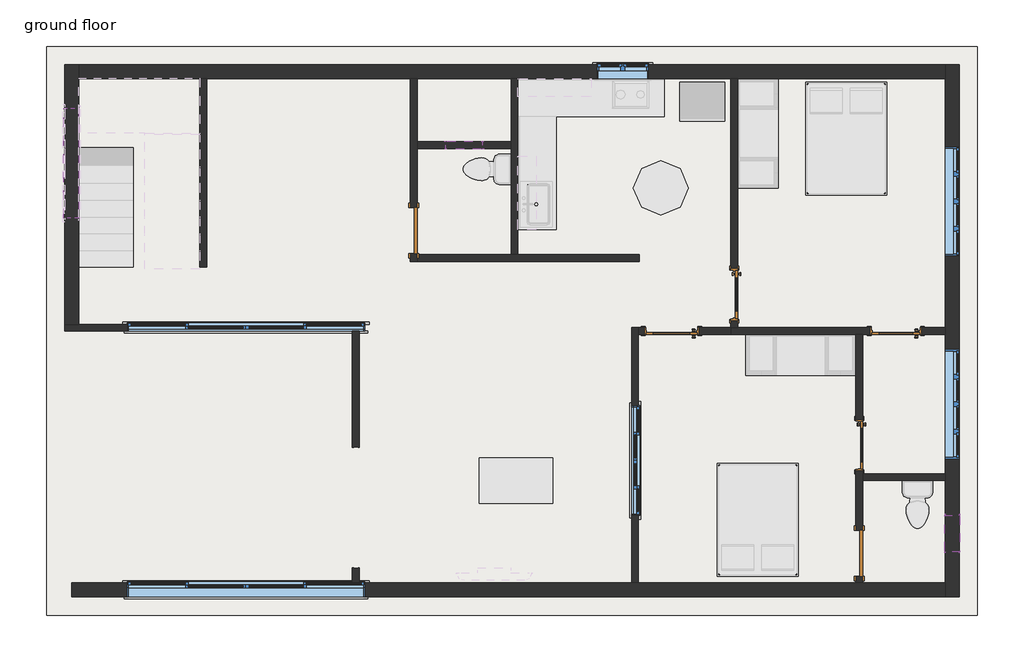
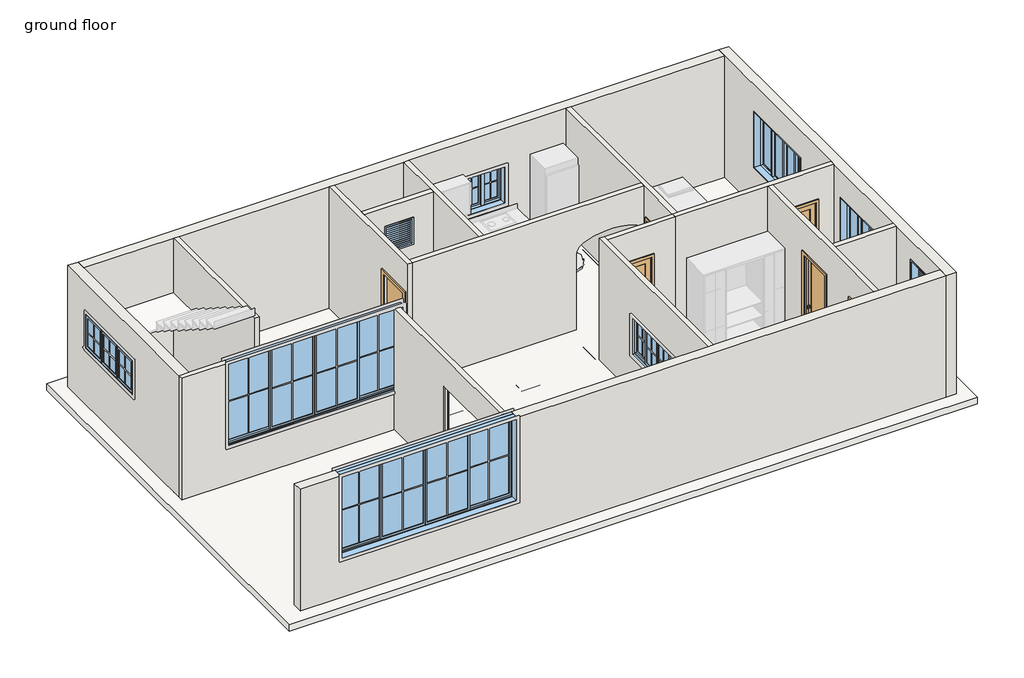
# One storey, part 1 of 2: 17 walls, 9 windows, 7 beams, 6 doors, 1 slab.
"""IFC4 building model written with IfcOpenShell, lengths in millimetres."""

from ifc_helpers import new_model, si_unit, point, frame, origin, place, context, project, spatial, polyline, ellipse_curve, trimmed, outline, extrude, faceted_brep, transform, mapped, element, save
from ifc_brep_helpers import plane_surface, extruded_surface, advanced_brep
from components import door_643e272e, door_51292941, door_214872d5, window_33d4544c, window_339605e1, window_5487fb6d, window_d39e7ecb, window_f2d8fef0, window_cbca41e3, window_8ea0b4a1, window_cd2bb1e7

model = new_model("IFC4")

# Units and contexts
model_context = context("Model", 3, world=origin())
ifc_project = project(units=[si_unit("LENGTHUNIT", "METRE", prefix="MILLI")], contexts=[model_context])

# Site, building, storey
site = spatial("IfcSite", under=ifc_project)
building = spatial("IfcBuilding", under=site)
storey = spatial("IfcBuildingStorey", under=building, Name="ground floor", Elevation=609.6)

# Beams
placement = place(None, origin())
element("IfcBeam", 1, ObjectType="Concrete-Rectangular Beam", at=placement, inside=storey, context=model_context, shape_type="Brep", body=[
    faceted_brep([(-12452.868339, 913.093496, 609.6), (-12452.868339, 684.493496, 609.6), (-8179.318339, 684.493496, 609.6), (-8179.318339, 913.093496, 609.6), (-12452.868339, 913.093496, 304.8), (-8179.318339, 913.093496, 304.8), (-12452.868339, 684.493496, 304.8), (-8179.318339, 684.493496, 304.8)], [[[0, 1, 2, 3]], [[4, 0, 3, 5]], [[6, 4, 5, 7]], [[1, 6, 7, 2]], [[1, 0, 4, 6]], [[3, 2, 7, 5]]]),
    faceted_brep([(1713.981661, 913.093496, 609.6), (1713.981661, 684.493496, 609.6), (1713.981661, 684.493496, 304.8), (1713.981661, 913.093496, 304.8), (-3226.216739, 684.493496, 609.6), (-3226.216739, 913.093496, 609.6), (-3226.216739, 913.093496, 304.8), (-3226.216739, 684.493496, 304.8), (469.381661, 913.093496, 609.6), (240.781661, 913.093496, 609.6), (-1613.418339, 913.093496, 609.6), (-1842.018339, 913.093496, 609.6), (469.381661, 913.093496, 304.8), (240.781661, 913.093496, 304.8), (-1613.418339, 913.093496, 304.8), (-1842.018339, 913.093496, 304.8)], [[[0, 1, 2, 3]], [[4, 5, 6, 7]], [[1, 0, 8, 9, 10, 11, 5, 4]], [[0, 3, 12, 13, 14, 15, 6, 5, 11, 10, 9, 8]], [[3, 2, 7, 6, 15, 14, 13, 12]], [[2, 1, 4, 7]]]),
    faceted_brep([(-7874.518339, 684.493496, 609.6), (-7874.518339, 913.093496, 609.6), (-7874.518339, 913.093496, 304.8), (-7874.518339, 684.493496, 304.8), (-3531.016739, 684.493496, 609.6), (-3531.016739, 913.093496, 609.6), (-5271.018339, 913.093496, 609.6), (-5499.618339, 913.093496, 609.6), (-6947.418339, 913.093496, 609.6), (-7176.018339, 913.093496, 609.6), (-3531.016739, 913.093496, 304.8), (-5271.018339, 913.093496, 304.8), (-5499.618339, 913.093496, 304.8), (-6947.418339, 913.093496, 304.8), (-7176.018339, 913.093496, 304.8), (-3531.016739, 684.493496, 304.8)], [[[0, 1, 2, 3]], [[1, 0, 4, 5, 6, 7, 8, 9]], [[2, 1, 9, 8, 7, 6, 5, 10, 11, 12, 13, 14]], [[3, 2, 14, 13, 12, 11, 10, 15]], [[0, 3, 15, 4]], [[5, 4, 15, 10]]]),
])
element("IfcBeam", 2, ObjectType="Concrete-Rectangular Beam", at=placement, inside=storey, context=model_context, shape_type="SweptSolid", body=[
    extrude(outline(polyline([(-12871.968339, 9244.293496), (-12643.368339, 9244.293496), (-12643.368339, 5415.243496), (-12871.968339, 5415.243496), (-12871.968339, 9244.293496)])), frame((0.0, 0.0, 304.8), z_axis=(0.0, 0.0, 1.0), x_axis=(1.0, 0.0, 0.0)), (0.0, 0.0, 1.0), 304.8),
])
element("IfcBeam", 3, ObjectType="Concrete-Rectangular Beam", at=placement, inside=storey, context=model_context, shape_type="Brep", body=[
    faceted_brep([(-10452.618339, 5110.443496, 609.6), (-10681.218339, 5110.443496, 609.6), (-10681.218339, 5110.443496, 304.8), (-10452.618339, 5110.443496, 304.8), (-10452.618339, 5148.543496, 609.6), (-10452.618339, 5377.143496, 609.6), (-10452.618339, 9282.393496, 609.6), (-10681.218339, 9282.393496, 609.6), (-10681.218339, 5377.143496, 609.6), (-10681.218339, 5148.543496, 609.6), (-10681.218339, 9282.393496, 304.8), (-10681.218339, 5377.143496, 304.8), (-10681.218339, 5148.543496, 304.8), (-10452.618339, 9282.393496, 304.8), (-10452.618339, 5377.143496, 304.8), (-10452.618339, 5148.543496, 304.8)], [[[0, 1, 2, 3]], [[1, 0, 4, 5, 6, 7, 8, 9]], [[2, 1, 9, 8, 7, 10, 11, 12]], [[3, 2, 12, 11, 10, 13, 14, 15]], [[0, 3, 15, 14, 13, 6, 5, 4]], [[7, 6, 13, 10]]]),
])
element("IfcBeam", 4, ObjectType="Concrete-Rectangular Beam", at=placement, inside=storey, context=model_context, shape_type="Brep", body=[
    faceted_brep([(-8274.568339, 5148.543496, 609.6), (-8274.568339, 5339.043496, 609.6), (-7969.768339, 5339.043496, 609.6), (-7969.768339, 5148.543496, 609.6), (-7912.618339, 5148.543496, 609.6), (-7912.618339, 5224.743496, 609.6), (-7912.618339, 5377.143496, 609.6), (-10452.618339, 5377.143496, 609.6), (-10452.618339, 5148.543496, 609.6), (-7969.768339, 5148.543496, 304.8), (-7912.618339, 5148.543496, 304.8), (-8274.568339, 5339.043496, 304.8), (-8274.568339, 5148.543496, 304.8), (-10452.618339, 5148.543496, 304.8), (-10452.618339, 5377.143496, 304.8), (-7912.618339, 5377.143496, 304.8), (-7912.618339, 5224.743496, 304.8), (-7969.768339, 5339.043496, 304.8)], [[[0, 1, 2, 3, 4, 5, 6, 7, 8]], [[3, 9, 10, 4]], [[11, 12, 13, 14, 15, 16, 10, 9, 17]], [[6, 15, 14, 7]], [[11, 1, 0, 12]], [[17, 2, 1, 11]], [[2, 17, 9, 3]], [[8, 7, 14, 13]], [[6, 5, 4, 10, 16, 15]], [[12, 0, 8, 13]]]),
    faceted_brep([(-12643.368339, 5148.543496, 609.6), (-12643.368339, 5377.143496, 609.6), (-12643.368339, 5377.143496, 304.8), (-12643.368339, 5148.543496, 304.8), (-10681.218339, 5377.143496, 609.6), (-10681.218339, 5148.543496, 609.6), (-10681.218339, 5148.543496, 304.8), (-10681.218339, 5377.143496, 304.8)], [[[0, 1, 2, 3]], [[4, 5, 6, 7]], [[1, 0, 5, 4]], [[3, 2, 7, 6]], [[2, 1, 4, 7]], [[0, 3, 6, 5]]]),
])
element("IfcBeam", 5, ObjectType="Concrete-Rectangular Beam", at=placement, inside=storey, context=model_context, shape_type="Brep", body=[
    faceted_brep([(-7912.618339, 5148.543496, 609.6), (-7969.768339, 5148.543496, 609.6), (-7969.768339, 5110.443496, 609.6), (-8141.218339, 5110.443496, 609.6), (-8141.218339, 913.093496, 609.6), (-7912.618339, 913.093496, 609.6), (-7912.618339, 4996.143496, 609.6), (-7912.618339, 5148.543496, 304.8), (-7912.618339, 913.093496, 304.8), (-7912.618339, 4996.143496, 304.8), (-7969.768339, 5148.543496, 304.8), (-8141.218339, 913.093496, 304.8), (-8141.218339, 5110.443496, 304.8), (-7969.768339, 5110.443496, 304.8)], [[[0, 1, 2, 3, 4, 5, 6]], [[7, 0, 6, 5, 8, 9]], [[10, 7, 9, 8, 11, 12, 13]], [[3, 12, 11, 4]], [[0, 7, 10, 1]], [[2, 13, 12, 3]], [[13, 2, 1, 10]], [[5, 4, 11, 8]]]),
])
element("IfcBeam", 6, ObjectType="Concrete-Rectangular Beam", at=placement, inside=storey, context=model_context, shape_type="Brep", body=[
    faceted_brep([(-6947.418339, 9282.393496, 609.6), (-7176.018339, 9282.393496, 609.6), (-7176.018339, 5224.743496, 609.6), (-7176.018339, 4996.143496, 609.6), (-7176.018339, 913.093496, 609.6), (-6947.418339, 913.093496, 609.6), (-6947.418339, 4996.143496, 609.6), (-6947.418339, 5224.743496, 609.6), (-6947.418339, 6215.343496, 609.6), (-6947.418339, 6443.943496, 609.6), (-6947.418339, 8094.943496, 609.6), (-6947.418339, 8323.543496, 609.6), (-7176.018339, 9282.393496, 304.8), (-7176.018339, 5224.743496, 304.8), (-7176.018339, 4996.143496, 304.8), (-7176.018339, 913.093496, 304.8), (-6947.418339, 9282.393496, 304.8), (-6947.418339, 8323.543496, 304.8), (-6947.418339, 8094.943496, 304.8), (-6947.418339, 6443.943496, 304.8), (-6947.418339, 6215.343496, 304.8), (-6947.418339, 5224.743496, 304.8), (-6947.418339, 4996.143496, 304.8), (-6947.418339, 913.093496, 304.8)], [[[0, 1, 2, 3, 4, 5, 6, 7, 8, 9, 10, 11]], [[1, 12, 13, 14, 15, 4, 3, 2]], [[12, 16, 17, 18, 19, 20, 21, 22, 23, 15, 14, 13]], [[16, 0, 11, 10, 9, 8, 7, 6, 5, 23, 22, 21, 20, 19, 18, 17]], [[1, 0, 16, 12]], [[5, 4, 15, 23]]]),
])
element("IfcBeam", 7, ObjectType="Concrete-Rectangular Beam", at=placement, inside=storey, context=model_context, shape_type="Brep", body=[
    faceted_brep([(-5271.018339, 9282.393496, 609.6), (-5499.618339, 9282.393496, 609.6), (-5499.618339, 8323.543496, 609.6), (-5499.618339, 8094.943496, 609.6), (-5499.618339, 6443.943496, 609.6), (-5499.618339, 6215.343496, 609.6), (-5499.618339, 5224.743496, 609.6), (-5499.618339, 4996.143496, 609.6), (-5499.618339, 913.093496, 609.6), (-5271.018339, 913.093496, 609.6), (-5271.018339, 4996.143496, 609.6), (-5271.018339, 5224.743496, 609.6), (-5271.018339, 6215.343496, 609.6), (-5271.018339, 6443.943496, 609.6), (-5499.618339, 9282.393496, 304.8), (-5499.618339, 8323.543496, 304.8), (-5499.618339, 8094.943496, 304.8), (-5499.618339, 6443.943496, 304.8), (-5499.618339, 6215.343496, 304.8), (-5499.618339, 5224.743496, 304.8), (-5499.618339, 4996.143496, 304.8), (-5499.618339, 913.093496, 304.8), (-5271.018339, 9282.393496, 304.8), (-5271.018339, 6443.943496, 304.8), (-5271.018339, 6215.343496, 304.8), (-5271.018339, 5224.743496, 304.8), (-5271.018339, 4996.143496, 304.8), (-5271.018339, 913.093496, 304.8)], [[[0, 1, 2, 3, 4, 5, 6, 7, 8, 9, 10, 11, 12, 13]], [[1, 14, 15, 16, 17, 18, 19, 20, 21, 8, 7, 6, 5, 4, 3, 2]], [[14, 22, 23, 24, 25, 26, 27, 21, 20, 19, 18, 17, 16, 15]], [[22, 0, 13, 12, 11, 10, 9, 27, 26, 25, 24, 23]], [[1, 0, 22, 14]], [[9, 8, 21, 27]]]),
])

# Doors
door_shape = door_643e272e(model_context)
element("IfcDoor", 8, ObjectType="Door-Interior-Single-1_Panel-Wood : 32\" x 84\"", at=placement, inside=storey, context=model_context, shape_type="MappedRepresentation", body=[
    mapped(door_shape, transform((-1724.543339, 5720.043496, 609.6), x_axis=(0.0, -1.0, 0.0), y_axis=(1.0, 0.0, 0.0), z_axis=(0.0, 0.0, 1.0))),
])
element("IfcDoor", 9, ObjectType="Door-Interior-Single-1_Panel-Wood : 32\" x 84\"", at=placement, inside=storey, context=model_context, shape_type="MappedRepresentation", body=[
    mapped(door_shape, transform((358.256661, 3211.793496, 609.6), x_axis=(0.0, -1.0, 0.0), y_axis=(1.0, 0.0, 0.0), z_axis=(0.0, 0.0, 1.0))),
])
element("IfcDoor", 10, ObjectType="Door-Interior-Single-1_Panel-Wood : 32\" x 84\"", at=placement, inside=storey, context=model_context, shape_type="MappedRepresentation", body=[
    mapped(door_shape, transform((964.681661, 5107.268496, 609.6), x_axis=(-1.0, 0.0, 0.0), y_axis=(0.0, -1.0, 0.0), z_axis=(0.0, 0.0, 1.0))),
])
door_2_shape = door_51292941(model_context)
element("IfcDoor", 11, ObjectType="Door-Interior-Single-1_Panel-Wood : 34\" x 84\"", at=placement, inside=storey, context=model_context, shape_type="MappedRepresentation", body=[
    mapped(door_2_shape, transform((-2769.016739, 5107.268496, 609.6), x_axis=(-1.0, 0.0, 0.0), y_axis=(0.0, -1.0, 0.0), z_axis=(0.0, 0.0, 1.0))),
])
door_3_shape = door_214872d5(model_context)
element("IfcDoor", 12, ObjectType="Single-Flush : 30\" x 84\"", at=placement, inside=storey, context=model_context, shape_type="MappedRepresentation", body=[
    mapped(door_3_shape, transform((355.081661, 1408.393496, 609.6), x_axis=(0.0, -1.0, 0.0), y_axis=(1.0, 0.0, 0.0), z_axis=(0.0, 0.0, 1.0))),
])
element("IfcDoor", 13, ObjectType="Single-Flush : 30\" x 84\"", at=placement, inside=storey, context=model_context, shape_type="MappedRepresentation", body=[
    mapped(door_3_shape, transform((-7061.718339, 6786.843496, 609.6), x_axis=(0.0, -1.0, 0.0), y_axis=(1.0, 0.0, 0.0), z_axis=(0.0, 0.0, 1.0))),
])

# Slab
element("IfcSlab", 14, ObjectType="Generic - 6\"", at=placement, inside=storey, context=model_context, shape_type="SweptSolid", body=[
    extrude(outline(polyline([(2323.581661, 9853.893496), (2323.581661, 379.693496), (-13176.768339, 379.693496), (-13176.768339, 9853.893496), (2323.581661, 9853.893496)])), frame((0.0, 0.0, 457.2), z_axis=(0.0, 0.0, 1.0), x_axis=(1.0, 0.0, 0.0)), (0.0, 0.0, 1.0), 152.4),
])

# Walls
element("IfcWall", 15, ObjectType="Generic - 4.5\"", at=placement, inside=storey, context=model_context, shape_type="SweptSolid", body=[
    extrude(outline(polyline([(-10624.068339, 6177.243496), (-10624.068339, 9320.493496), (-10509.768339, 9320.493496), (-10509.768339, 6177.243496), (-10624.068339, 6177.243496)])), frame((0.0, 0.0, 609.6), z_axis=(0.0, 0.0, 1.0), x_axis=(1.0, 0.0, 0.0)), (0.0, 0.0, 1.0), 2895.6),
])
element("IfcWall", 16, ObjectType="Generic - 4.5\"", at=placement, inside=storey, context=model_context, shape_type="Brep", body=[
    faceted_brep([(-7118.868339, 6405.843496, 2743.2), (-7118.868339, 6405.843496, 609.6), (-7118.868339, 6272.493496, 609.6), (-7118.868339, 6272.493496, 3505.2), (-7118.868339, 9320.493496, 3505.2), (-7118.868339, 9320.493496, 609.6), (-7118.868339, 7167.843496, 609.6), (-7118.868339, 7167.843496, 2743.2), (-7004.568339, 6272.493496, 609.6), (-7004.568339, 6386.793496, 609.6), (-7004.568339, 6405.843496, 609.6), (-7004.568339, 6405.843496, 2743.2), (-7004.568339, 7167.843496, 2743.2), (-7004.568339, 7167.843496, 609.6), (-7004.568339, 8152.093496, 609.6), (-7004.568339, 8266.393496, 609.6), (-7004.568339, 9320.493496, 609.6), (-7004.568339, 9320.493496, 3505.2), (-7004.568339, 8266.393496, 3505.2), (-7004.568339, 8152.093496, 3505.2), (-7004.568339, 6386.793496, 3505.2), (-7004.568339, 6272.493496, 3505.2)], [[[0, 1, 2, 3, 4, 5, 6, 7]], [[8, 9, 10, 11, 12, 13, 14, 15, 16, 17, 18, 19, 20, 21]], [[6, 5, 16, 15, 14, 13]], [[2, 1, 10, 9, 8]], [[4, 3, 21, 20, 19, 18, 17]], [[3, 2, 8, 21]], [[5, 4, 17, 16]], [[11, 10, 1, 0]], [[12, 11, 0, 7]], [[13, 12, 7, 6]]]),
])
element("IfcWall", 17, ObjectType="Generic - 4.5\"", at=placement, inside=storey, context=model_context, shape_type="Brep", body=[
    faceted_brep([(-5442.468339, 9320.493496, 609.6), (-5442.468339, 8266.393496, 609.6), (-5442.468339, 8152.093496, 609.6), (-5442.468339, 6386.793496, 609.6), (-5442.468339, 6386.793496, 3505.2), (-5442.468339, 8152.093496, 3505.2), (-5442.468339, 8266.393496, 3505.2), (-5442.468339, 9320.493496, 3505.2), (-5328.168339, 9320.493496, 609.6), (-5328.168339, 9320.493496, 3505.2), (-5328.168339, 6386.793496, 3505.2), (-5328.168339, 6386.793496, 609.6)], [[[0, 1, 2, 3, 4, 5, 6, 7]], [[8, 9, 10, 11]], [[3, 2, 1, 0, 8, 11]], [[7, 6, 5, 4, 10, 9]], [[4, 3, 11, 10]], [[0, 7, 9, 8]]]),
])
element("IfcWall", 18, ObjectType="Generic - 4.5\"", at=placement, inside=storey, context=model_context, shape_type="Brep", body=[
    faceted_brep([(-1784.868339, 5167.593496, 3505.2), (-1784.868339, 6272.493496, 3505.2), (-1784.868339, 6386.793496, 3505.2), (-1784.868339, 9320.493496, 3505.2), (-1784.868339, 9320.493496, 609.6), (-1784.868339, 6386.793496, 609.6), (-1784.868339, 6272.493496, 609.6), (-1784.868339, 6151.843496, 609.6), (-1784.868339, 6151.843496, 2768.6), (-1784.868339, 5288.243496, 2768.6), (-1784.868339, 5288.243496, 609.6), (-1784.868339, 5167.593496, 609.6), (-1670.568339, 9320.493496, 3505.2), (-1670.568339, 5167.593496, 3505.2), (-1670.568339, 5167.593496, 609.6), (-1670.568339, 5288.243496, 609.6), (-1670.568339, 5288.243496, 2768.6), (-1670.568339, 6151.843496, 2768.6), (-1670.568339, 6151.843496, 609.6), (-1670.568339, 9320.493496, 609.6)], [[[0, 1, 2, 3, 4, 5, 6, 7, 8, 9, 10, 11]], [[12, 13, 14, 15, 16, 17, 18, 19]], [[14, 11, 10, 15]], [[4, 19, 18, 7, 6, 5]], [[3, 2, 1, 0, 13, 12]], [[0, 11, 14, 13]], [[4, 3, 12, 19]], [[9, 16, 15, 10]], [[16, 9, 8, 17]], [[17, 8, 7, 18]]]),
])
element("IfcWall", 19, ObjectType="Generic - 4.5\"", at=placement, inside=storey, context=model_context, shape_type="Brep", body=[
    faceted_brep([(-1784.868339, 5167.593496, 3505.2), (-1670.568339, 5167.593496, 3505.2), (1790.181661, 5167.593496, 3505.2), (1790.181661, 5167.593496, 609.6), (1396.481661, 5167.593496, 609.6), (1396.481661, 5167.593496, 2768.6), (532.881661, 5167.593496, 2768.6), (532.881661, 5167.593496, 609.6), (-1670.568339, 5167.593496, 609.6), (-1784.868339, 5167.593496, 609.6), (1790.181661, 5053.293496, 3505.2), (412.231661, 5053.293496, 3505.2), (297.931661, 5053.293496, 3505.2), (-1784.868339, 5053.293496, 3505.2), (-1784.868339, 5053.293496, 609.6), (297.931661, 5053.293496, 609.6), (412.231661, 5053.293496, 609.6), (532.881661, 5053.293496, 609.6), (532.881661, 5053.293496, 2768.6), (1396.481661, 5053.293496, 2768.6), (1396.481661, 5053.293496, 609.6), (1790.181661, 5053.293496, 609.6)], [[[0, 1, 2, 3, 4, 5, 6, 7, 8, 9]], [[10, 11, 12, 13, 14, 15, 16, 17, 18, 19, 20, 21]], [[3, 21, 20, 4]], [[14, 9, 8, 7, 17, 16, 15]], [[2, 1, 0, 13, 12, 11, 10]], [[3, 2, 10, 21]], [[0, 9, 14, 13]], [[6, 18, 17, 7]], [[18, 6, 5, 19]], [[19, 5, 4, 20]]]),
])
element("IfcWall", 20, ObjectType="Generic - 4.5\"", at=placement, inside=storey, context=model_context, shape_type="AdvancedBrep", body=[
    advanced_brep(
    [(-1784.868339, 6272.493496, 3505.2), (-7004.568339, 6272.493496, 3505.2), (-7004.568339, 6272.493496, 609.6), (-3308.868339, 6272.493496, 609.6), (-3308.868339, 6272.493496, 2438.4), (-1784.868339, 6272.493496, 2438.4), (-7004.568339, 6386.793496, 3505.2), (-5442.468339, 6386.793496, 3505.2), (-5328.168339, 6386.793496, 3505.2), (-1784.868339, 6386.793496, 3505.2), (-1784.868339, 6386.793496, 2438.4), (-3308.868339, 6386.793496, 2438.4), (-3308.868339, 6386.793496, 609.6), (-5328.168339, 6386.793496, 609.6), (-5442.468339, 6386.793496, 609.6), (-7004.568339, 6386.793496, 609.6)],
    [
        (0, 1),
        (1, 2),
        (2, 3),
        (3, 4),
        (4, 5, ellipse_curve(frame((-2546.868339, 6272.493496, 2438.4), z_axis=(0.0, 1.0, 0.0), x_axis=(1.0, 0.0, 0.0)), 762.0, 304.8)),
        (5, 0),
        (6, 7),
        (7, 8),
        (8, 9),
        (9, 10),
        (10, 11, ellipse_curve(frame((-2546.868339, 6386.793496, 2438.4), z_axis=(0.0, -1.0, 0.0), x_axis=(1.0, 0.0, 0.0)), 762.0, 304.8)),
        (11, 12),
        (12, 13),
        (13, 14),
        (14, 15),
        (15, 6),
        (2, 15),
        (12, 3),
        (0, 9),
        (6, 1),
        (5, 10),
        (4, 11),
    ],
    [
        plane_surface(frame((-7061.718339, 6272.493496, 609.6), z_axis=(0.0, -1.0, 0.0), x_axis=(1.0, 0.0, 0.0))),
        plane_surface(frame((-7061.718339, 6386.793496, 609.6), z_axis=(0.0, 1.0, 0.0), x_axis=(-1.0, 0.0, 0.0))),
        plane_surface(frame((-7061.718339, 6272.493496, 609.6), z_axis=(0.0, 0.0, -1.0), x_axis=(0.0, 1.0, 0.0))),
        plane_surface(frame((-1727.718339, 6272.493496, 3505.2), z_axis=(0.0, 0.0, 1.0), x_axis=(0.0, 1.0, 0.0))),
        plane_surface(frame((-7004.568339, 9377.643496, 609.6), z_axis=(-1.0, 0.0, 0.0), x_axis=(0.0, 1.0, 0.0))),
        plane_surface(frame((-1784.868339, 9377.643496, 609.6), z_axis=(1.0, 0.0, 0.0), x_axis=(0.0, -1.0, 0.0))),
        extruded_surface(trimmed(ellipse_curve(frame((-2546.868339, 7796.493496, 2438.4), z_axis=(0.0, -1.0, 0.0), x_axis=(1.0, 0.0, 0.0)), 762.0, 304.8), [point((-1784.868339, 7796.493496, 2438.4))], [point((-3308.868339, 7796.493496, 2438.4))], True, "CARTESIAN"), (0.0, 3047.999999999999, 0.0), 3047.999999999999),
        plane_surface(frame((-3308.868339, 4748.493496, 2438.4), z_axis=(1.0, 0.0, 0.0), x_axis=(0.0, 1.0, 0.0))),
    ],
    [
        (0, [[1, 2, 3, 4, 5, 6]]),
        (1, [[7, 8, 9, 10, 11, 12, 13, 14, 15, 16]]),
        (2, [[17, -15, -14, -13, 18, -3]]),
        (3, [[-1, 19, -9, -8, -7, 20]]),
        (4, [[-2, -20, -16, -17]]),
        (5, [[-19, -6, 21, -10]]),
        (6, [[22, -11, -21, -5]]),
        (7, [[-22, -4, -18, -12]]),
    ],
),
])
element("IfcWall", 21, ObjectType="Generic - 4.5\"", at=placement, inside=storey, context=model_context, shape_type="Brep", body=[
    faceted_brep([(297.931661, 913.093496, 3505.2), (297.931661, 5053.293496, 3505.2), (297.931661, 5053.293496, 609.6), (297.931661, 3643.593496, 609.6), (297.931661, 3643.593496, 2768.6), (297.931661, 2779.993496, 2768.6), (297.931661, 2779.993496, 609.6), (297.931661, 1789.393496, 609.6), (297.931661, 1789.393496, 2743.2), (297.931661, 1027.393496, 2743.2), (297.931661, 1027.393496, 609.6), (297.931661, 913.093496, 609.6), (412.231661, 5053.293496, 3505.2), (412.231661, 2735.543496, 3505.2), (412.231661, 2621.243496, 3505.2), (412.231661, 913.093496, 3505.2), (412.231661, 913.093496, 609.6), (412.231661, 1027.393496, 609.6), (412.231661, 1027.393496, 2743.2), (412.231661, 1789.393496, 2743.2), (412.231661, 1789.393496, 609.6), (412.231661, 2621.243496, 609.6), (412.231661, 2735.543496, 609.6), (412.231661, 2779.993496, 609.6), (412.231661, 2779.993496, 2768.6), (412.231661, 3643.593496, 2768.6), (412.231661, 3643.593496, 609.6), (412.231661, 5053.293496, 609.6)], [[[0, 1, 2, 3, 4, 5, 6, 7, 8, 9, 10, 11]], [[12, 13, 14, 15, 16, 17, 18, 19, 20, 21, 22, 23, 24, 25, 26, 27]], [[2, 27, 26, 3]], [[16, 11, 10, 17]], [[20, 7, 6, 23, 22, 21]], [[1, 0, 15, 14, 13, 12]], [[2, 1, 12, 27]], [[0, 11, 16, 15]], [[18, 17, 10, 9]], [[19, 18, 9, 8]], [[20, 19, 8, 7]], [[5, 24, 23, 6]], [[24, 5, 4, 25]], [[25, 4, 3, 26]]]),
])
element("IfcWall", 22, ObjectType="Generic - 4.5\"", at=placement, inside=storey, context=model_context, shape_type="SweptSolid", body=[
    extrude(outline(polyline([(1790.181661, 2621.243496), (412.231661, 2621.243496), (412.231661, 2735.543496), (1790.181661, 2735.543496), (1790.181661, 2621.243496)])), frame((0.0, 0.0, 609.6), z_axis=(0.0, 0.0, 1.0), x_axis=(1.0, 0.0, 0.0)), (0.0, 0.0, 1.0), 2895.6),
])
element("IfcWall", 23, ObjectType="Generic - 4.5\"", at=placement, inside=storey, context=model_context, shape_type="Brep", body=[
    faceted_brep([(-3435.766739, 5167.593496, 609.6), (-3435.766739, 913.093496, 609.6), (-3435.766739, 913.093496, 3505.2), (-3435.766739, 5167.593496, 3505.2), (-3435.766739, 2040.218496, 2438.4), (-3435.766739, 2040.218496, 1524.0), (-3435.766739, 3869.018496, 1524.0), (-3435.766739, 3869.018496, 2438.4), (-3321.466739, 5167.593496, 609.6), (-3321.466739, 5167.593496, 3505.2), (-3321.466739, 5053.293496, 3505.2), (-3321.466739, 913.093496, 3505.2), (-3321.466739, 913.093496, 609.6), (-3321.466739, 5053.293496, 609.6), (-3321.466739, 2040.218496, 2438.4), (-3321.466739, 3869.018496, 2438.4), (-3321.466739, 3869.018496, 1524.0), (-3321.466739, 2040.218496, 1524.0)], [[[0, 1, 2, 3], [4, 5, 6, 7]], [[8, 9, 10, 11, 12, 13], [14, 15, 16, 17]], [[1, 0, 8, 13, 12]], [[3, 2, 11, 10, 9]], [[2, 1, 12, 11]], [[0, 3, 9, 8]], [[5, 4, 14, 17]], [[6, 5, 17, 16]], [[7, 6, 16, 15]], [[4, 7, 15, 14]]]),
])
element("IfcWall", 24, ObjectType="Generic - 4.5\"", at=placement, inside=storey, context=model_context, shape_type="Brep", body=[
    faceted_brep([(-8084.068339, 913.093496, 609.6), (-8084.068339, 913.093496, 3505.2), (-8084.068339, 5110.443496, 3505.2), (-8084.068339, 5110.443496, 1524.0), (-8084.068339, 5224.743496, 1524.0), (-8084.068339, 5224.743496, 609.6), (-8084.068339, 5110.443496, 609.6), (-8084.068339, 3170.393496, 609.6), (-8084.068339, 3170.393496, 2818.6), (-8084.068339, 1170.393496, 2818.6), (-8084.068339, 1170.393496, 609.6), (-7969.768339, 913.093496, 3505.2), (-7969.768339, 913.093496, 609.6), (-7969.768339, 1170.393496, 609.6), (-7969.768339, 1170.393496, 2818.6), (-7969.768339, 3170.393496, 2818.6), (-7969.768339, 3170.393496, 609.6), (-7969.768339, 5224.743496, 609.6), (-7969.768339, 5224.743496, 1524.0), (-7969.768339, 5110.443496, 1524.0), (-7969.768339, 5110.443496, 3505.2), (-8059.7683389, 1170.393496, 609.6), (-8059.7683389, 1155.393496, 609.6), (-7989.7683389, 1155.393496, 609.6), (-7989.7683389, 1170.393496, 609.6), (-7989.7683389, 3170.393496, 609.6), (-7989.7683389, 3185.393496, 609.6), (-8059.7683389, 3185.393496, 609.6), (-8059.7683389, 3170.393496, 609.6), (-7989.7683389, 1170.393496, 2818.6), (-7989.7683389, 3170.393496, 2818.6), (-8059.7683389, 3170.393496, 2818.6), (-8059.7683389, 1170.393496, 2818.6), (-8059.7683389, 3185.393496, 2833.6), (-8059.7683389, 1155.393496, 2833.6), (-7989.7683389, 1155.393496, 2833.6), (-7989.7683389, 3185.393496, 2833.6)], [[[0, 1, 2, 3, 4, 5, 6, 7, 8, 9, 10]], [[11, 12, 13, 14, 15, 16, 17, 18, 19, 20]], [[12, 0, 10, 21, 22, 23, 24, 13]], [[5, 17, 16, 25, 26, 27, 28, 7, 6]], [[1, 11, 20, 2]], [[1, 0, 12, 11]], [[17, 5, 4, 18]], [[29, 30, 15, 14]], [[31, 32, 9, 8]], [[28, 31, 8, 7]], [[32, 21, 10, 9]], [[32, 31, 28, 27, 33, 34, 22, 21]], [[22, 34, 35, 23]], [[30, 29, 24, 23, 35, 36, 26, 25]], [[24, 29, 14, 13]], [[30, 25, 16, 15]], [[33, 27, 26, 36]], [[34, 33, 36, 35]], [[19, 3, 2, 20]], [[3, 19, 18, 4]]]),
])
element("IfcWall", 25, ObjectType="Generic - 4.5\"", at=placement, inside=storey, context=model_context, shape_type="Brep", body=[
    faceted_brep([(-8084.068339, 5224.743496, 609.6), (-12643.368339, 5224.743496, 609.6), (-12871.968339, 5224.743496, 609.6), (-12871.968339, 5224.743496, 3505.2), (-12643.368339, 5224.743496, 3505.2), (-11836.918339, 5224.743496, 3505.2), (-11836.918339, 5224.743496, 1524.0), (-8084.068339, 5224.743496, 1524.0), (-12871.968339, 5110.443496, 609.6), (-8084.068339, 5110.443496, 609.6), (-8084.068339, 5110.443496, 1524.0), (-11836.918339, 5110.443496, 1524.0), (-11836.918339, 5110.443496, 3505.2), (-12871.968339, 5110.443496, 3505.2)], [[[0, 1, 2, 3, 4, 5, 6, 7]], [[8, 9, 10, 11, 12, 13]], [[2, 1, 0, 9, 8]], [[3, 13, 12, 5, 4]], [[9, 0, 7, 10]], [[3, 2, 8, 13]], [[6, 11, 10, 7]], [[11, 6, 5, 12]]]),
])
element("IfcWall", 26, ObjectType="Generic - 4.5\"", at=placement, inside=storey, context=model_context, shape_type="SweptSolid", body=[
    extrude(outline(polyline([(3505.2, -1784.868339), (3505.2, -3321.466739), (609.6, -3321.466739), (609.6, -3226.216739), (2768.6, -3226.216739), (2768.6, -2311.816739), (609.6, -2311.816739), (609.6, -1784.868339), (3505.2, -1784.868339)])), frame((0.0, 5053.293496, 0.0), z_axis=(0.0, 1.0, 0.0), x_axis=(0.0, 0.0, 1.0)), (0.0, 0.0, 1.0), 114.3),
])
element("IfcWall", 27, ObjectType="Generic - 4.5\"", at=placement, inside=storey, context=model_context, shape_type="SweptSolid", body=[
    extrude(outline(polyline([(609.6, -7004.568339), (609.6, -5442.468339), (3505.2, -5442.468339), (3505.2, -7004.568339), (609.6, -7004.568339)]), holes=[polyline([(3048.0, -6528.318339), (3048.0, -5918.718339), (2438.4, -5918.718339), (2438.4, -6528.318339), (3048.0, -6528.318339)])]), frame((0.0, 8152.093496, 0.0), z_axis=(0.0, 1.0, 0.0), x_axis=(0.0, 0.0, 1.0)), (0.0, 0.0, 1.0), 114.3),
])
element("IfcWall", 28, ObjectType="Generic - 9\"", at=placement, inside=storey, context=model_context, shape_type="Brep", body=[
    faceted_brep([(1790.181661, 9549.093496, 609.6), (1790.181661, 9320.493496, 609.6), (1790.181661, 5167.593496, 609.6), (1790.181661, 5053.293496, 609.6), (1790.181661, 2735.543496, 609.6), (1790.181661, 2621.243496, 609.6), (1790.181661, 913.093496, 609.6), (1790.181661, 684.493496, 609.6), (1790.181661, 684.493496, 3505.2), (1790.181661, 913.093496, 3505.2), (1790.181661, 2621.243496, 3505.2), (1790.181661, 2735.543496, 3505.2), (1790.181661, 5053.293496, 3505.2), (1790.181661, 5167.593496, 3505.2), (1790.181661, 9320.493496, 3505.2), (1790.181661, 9549.093496, 3505.2), (1790.181661, 6358.218496, 2870.2), (1790.181661, 6358.218496, 1524.0), (1790.181661, 8187.018496, 1524.0), (1790.181661, 8187.018496, 2870.2), (1790.181661, 2043.393496, 3048.0), (1790.181661, 1433.793496, 3048.0), (1790.181661, 1433.793496, 2438.4), (1790.181661, 2043.393496, 2438.4), (1790.181661, 2980.018496, 2870.2), (1790.181661, 2980.018496, 1524.0), (1790.181661, 4808.818496, 1524.0), (1790.181661, 4808.818496, 2870.2), (2018.781661, 9549.093496, 609.6), (2018.781661, 9549.093496, 3505.2), (2018.781661, 684.493496, 3505.2), (2018.781661, 684.493496, 609.6), (2018.781661, 6358.218496, 2870.2), (2018.781661, 8187.018496, 2870.2), (2018.781661, 8187.018496, 1524.0), (2018.781661, 6358.218496, 1524.0), (2018.781661, 2043.393496, 3048.0), (2018.781661, 2043.393496, 2438.4), (2018.781661, 1433.793496, 2438.4), (2018.781661, 1433.793496, 3048.0), (2018.781661, 2980.018496, 2870.2), (2018.781661, 4808.818496, 2870.2), (2018.781661, 4808.818496, 1524.0), (2018.781661, 2980.018496, 1524.0)], [[[0, 1, 2, 3, 4, 5, 6, 7, 8, 9, 10, 11, 12, 13, 14, 15], [16, 17, 18, 19], [20, 21, 22, 23], [24, 25, 26, 27]], [[28, 29, 30, 31], [32, 33, 34, 35], [36, 37, 38, 39], [40, 41, 42, 43]], [[7, 6, 5, 4, 3, 2, 1, 0, 28, 31]], [[15, 14, 13, 12, 11, 10, 9, 8, 30, 29]], [[0, 15, 29, 28]], [[8, 7, 31, 30]], [[17, 16, 32, 35]], [[18, 17, 35, 34]], [[19, 18, 34, 33]], [[16, 19, 33, 32]], [[37, 36, 20, 23]], [[38, 37, 23, 22]], [[39, 38, 22, 21]], [[36, 39, 21, 20]], [[25, 24, 40, 43]], [[26, 25, 43, 42]], [[27, 26, 42, 41]], [[24, 27, 41, 40]]]),
])
element("IfcWall", 29, ObjectType="Generic - 9\"", at=placement, inside=storey, context=model_context, shape_type="Brep", body=[
    faceted_brep([(1790.181661, 913.093496, 609.6), (412.231661, 913.093496, 609.6), (297.931661, 913.093496, 609.6), (-3321.466739, 913.093496, 609.6), (-3435.766739, 913.093496, 609.6), (-7969.768339, 913.093496, 609.6), (-8084.068339, 913.093496, 609.6), (-12757.668339, 913.093496, 609.6), (-12757.668339, 913.093496, 3505.2), (-11836.918339, 913.093496, 3505.2), (-11836.918339, 913.093496, 1524.0), (-7874.518339, 913.093496, 1524.0), (-7874.518339, 913.093496, 3505.2), (-3435.766739, 913.093496, 3505.2), (-3321.466739, 913.093496, 3505.2), (297.931661, 913.093496, 3505.2), (412.231661, 913.093496, 3505.2), (1790.181661, 913.093496, 3505.2), (-12757.668339, 684.493496, 609.6), (1790.181661, 684.493496, 609.6), (1790.181661, 684.493496, 3505.2), (-7874.518339, 684.493496, 3505.2), (-7874.518339, 684.493496, 1524.0), (-11836.918339, 684.493496, 1524.0), (-11836.918339, 684.493496, 3505.2), (-12757.668339, 684.493496, 3505.2)], [[[0, 1, 2, 3, 4, 5, 6, 7, 8, 9, 10, 11, 12, 13, 14, 15, 16, 17]], [[18, 19, 20, 21, 22, 23, 24, 25]], [[7, 6, 5, 4, 3, 2, 1, 0, 19, 18]], [[8, 7, 18, 25]], [[8, 25, 24, 9]], [[20, 17, 16, 15, 14, 13, 12, 21]], [[0, 17, 20, 19]], [[11, 22, 21, 12]], [[22, 11, 10, 23]], [[23, 10, 9, 24]]]),
])
element("IfcWall", 30, ObjectType="Generic - 9\"", at=placement, inside=storey, context=model_context, shape_type="Brep", body=[
    faceted_brep([(-12871.968339, 9549.093496, 609.6), (-12871.968339, 5224.743496, 609.6), (-12871.968339, 5224.743496, 3505.2), (-12871.968339, 9549.093496, 3505.2), (-12871.968339, 6996.393496, 2794.0), (-12871.968339, 6996.393496, 1981.2), (-12871.968339, 8825.193496, 1981.2), (-12871.968339, 8825.193496, 2794.0), (-12643.368339, 9549.093496, 609.6), (-12643.368339, 9549.093496, 3505.2), (-12643.368339, 9320.493496, 3505.2), (-12643.368339, 5224.743496, 3505.2), (-12643.368339, 5224.743496, 609.6), (-12643.368339, 9320.493496, 609.6), (-12643.368339, 6996.393496, 2794.0), (-12643.368339, 8825.193496, 2794.0), (-12643.368339, 8825.193496, 1981.2), (-12643.368339, 6996.393496, 1981.2)], [[[0, 1, 2, 3], [4, 5, 6, 7]], [[8, 9, 10, 11, 12, 13], [14, 15, 16, 17]], [[1, 0, 8, 13, 12]], [[3, 2, 11, 10, 9]], [[0, 3, 9, 8]], [[2, 1, 12, 11]], [[5, 4, 14, 17]], [[6, 5, 17, 16]], [[7, 6, 16, 15]], [[4, 7, 15, 14]]]),
])
element("IfcWall", 31, ObjectType="Generic - 9\"", at=placement, inside=storey, context=model_context, shape_type="Brep", body=[
    faceted_brep([(-12643.368339, 9320.493496, 609.6), (-10624.068339, 9320.493496, 609.6), (-10509.768339, 9320.493496, 609.6), (-7118.868339, 9320.493496, 609.6), (-7004.568339, 9320.493496, 609.6), (-5442.468339, 9320.493496, 609.6), (-5328.168339, 9320.493496, 609.6), (-1784.868339, 9320.493496, 609.6), (-1670.568339, 9320.493496, 609.6), (1790.181661, 9320.493496, 609.6), (1790.181661, 9320.493496, 3505.2), (-1670.568339, 9320.493496, 3505.2), (-1784.868339, 9320.493496, 3505.2), (-5328.168339, 9320.493496, 3505.2), (-5442.468339, 9320.493496, 3505.2), (-7004.568339, 9320.493496, 3505.2), (-7118.868339, 9320.493496, 3505.2), (-10509.768339, 9320.493496, 3505.2), (-10624.068339, 9320.493496, 3505.2), (-12643.368339, 9320.493496, 3505.2), (-3150.118339, 9320.493496, 2628.9), (-3150.118339, 9320.493496, 1714.5), (-4013.718339, 9320.493496, 1714.5), (-4013.718339, 9320.493496, 2628.9), (-12643.368339, 9549.093496, 609.6), (-12643.368339, 9549.093496, 3505.2), (1790.181661, 9549.093496, 3505.2), (1790.181661, 9549.093496, 609.6), (-3150.118339, 9549.093496, 2628.9), (-4013.718339, 9549.093496, 2628.9), (-4013.718339, 9549.093496, 1714.5), (-3150.118339, 9549.093496, 1714.5)], [[[0, 1, 2, 3, 4, 5, 6, 7, 8, 9, 10, 11, 12, 13, 14, 15, 16, 17, 18, 19], [20, 21, 22, 23]], [[24, 25, 26, 27], [28, 29, 30, 31]], [[9, 8, 7, 6, 5, 4, 3, 2, 1, 0, 24, 27]], [[19, 18, 17, 16, 15, 14, 13, 12, 11, 10, 26, 25]], [[10, 9, 27, 26]], [[0, 19, 25, 24]], [[21, 20, 28, 31]], [[22, 21, 31, 30]], [[23, 22, 30, 29]], [[20, 23, 29, 28]]]),
])

# Windows
window_shape = window_33d4544c(model_context)
element("IfcWindow", 32, ObjectType="Window-Awning-Triple-Horizontal : 72\" x 32\"", at=placement, inside=storey, context=model_context, shape_type="MappedRepresentation", body=[
    mapped(window_shape, transform((-12757.668339, 7910.793496, 1066.8), x_axis=(0.0, -1.0, 0.0), y_axis=(1.0, 0.0, 0.0), z_axis=(0.0, 0.0, 1.0))),
])
window_2_shape = window_339605e1(model_context)
element("IfcWindow", 33, ObjectType="Window-Casement-Double : 34\" x 36\"", at=placement, inside=storey, context=model_context, shape_type="MappedRepresentation", body=[
    mapped(window_2_shape, transform((-3581.918339, 9434.793496, 800.1), x_axis=(1.0, 0.0, 0.0), y_axis=(0.0, 1.0, 0.0), z_axis=(0.0, 0.0, 1.0))),
])
window_3_shape = window_5487fb6d(model_context)
element("IfcWindow", 34, ObjectType="Window-Casement-Multi-Sash-Horizontal : 72\" x 53\"", at=placement, inside=storey, context=model_context, shape_type="MappedRepresentation", body=[
    mapped(window_3_shape, transform((1904.481661, 7272.618496, 609.6), x_axis=(0.0, -1.0, 0.0), y_axis=(1.0, 0.0, 0.0), z_axis=(0.0, 0.0, 1.0))),
])
element("IfcWindow", 35, ObjectType="Window-Casement-Multi-Sash-Horizontal : 72\" x 53\"", at=placement, inside=storey, context=model_context, shape_type="MappedRepresentation", body=[
    mapped(window_3_shape, transform((1904.481661, 3894.418496, 609.6), x_axis=(0.0, -1.0, 0.0), y_axis=(1.0, 0.0, 0.0), z_axis=(0.0, 0.0, 1.0))),
])
window_4_shape = window_d39e7ecb(model_context)
element("IfcWindow", 36, ObjectType="Window-Louvers : 24\" x 24\"", at=placement, inside=storey, context=model_context, shape_type="MappedRepresentation", body=[
    mapped(window_4_shape, transform((-6223.518339, 8215.593496, 1524.0), x_axis=(1.0, 0.0, 0.0), y_axis=(0.0, 1.0, 0.0), z_axis=(0.0, 0.0, 1.0))),
])
window_5_shape = window_f2d8fef0(model_context)
element("IfcWindow", 37, ObjectType="Window-Louvers : 24\" x 24\"", at=placement, inside=storey, context=model_context, shape_type="MappedRepresentation", body=[
    mapped(window_5_shape, transform((1910.831661, 1738.593496, 1524.0), x_axis=(0.0, -1.0, 0.0), y_axis=(1.0, 0.0, 0.0), z_axis=(0.0, 0.0, 1.0))),
])
window_6_shape = window_cbca41e3(model_context)
element("IfcWindow", 38, ObjectType="Window-Sliding-Four : 156\" x 78\"", at=placement, inside=storey, context=model_context, shape_type="MappedRepresentation", body=[
    mapped(window_6_shape, transform((-9855.718339, 5171.403496, 609.6), x_axis=(1.0, 0.0, 0.0), y_axis=(0.0, 1.0, 0.0), z_axis=(0.0, 0.0, 1.0))),
])
window_7_shape = window_8ea0b4a1(model_context)
element("IfcWindow", 39, ObjectType="Window-Sliding-Four : 156\" x 78\"", at=placement, inside=storey, context=model_context, shape_type="MappedRepresentation", body=[
    mapped(window_7_shape, transform((-9855.718339, 802.603496, 609.6), x_axis=(1.0, 0.0, 0.0), y_axis=(0.0, 1.0, 0.0), z_axis=(0.0, 0.0, 1.0))),
])
window_8_shape = window_cd2bb1e7(model_context)
element("IfcWindow", 40, ObjectType="Window-Sliding-Four : 72\" x 36\"", at=placement, inside=storey, context=model_context, shape_type="MappedRepresentation", body=[
    mapped(window_8_shape, transform((-3374.806739, 2954.618496, 609.6), x_axis=(0.0, -1.0, 0.0), y_axis=(1.0, 0.0, 0.0), z_axis=(0.0, 0.0, 1.0))),
])

save(model, "model.ifc")

# Revit data of these elements
# Type "Concrete-Rectangular Beam"
#   Assembly Code = "B10"
#   Length [instance default] = 5 ft
#   b = 0.75 ft
#   h = 1 ft
#   Structural Material [instance default] = Concrete, Cast-in-Place gray
# Type "Door-Interior-Single-1_Panel-Wood : 32\" x 84\""
#   Type Mark = "8"
#   Assembly Code = "C1020300"
#   Analytic Construction = "Wooden"
#   Top Rail = 0.390625 ft
#   Thickness = 0.114583 ft
#   Thermal Resistance (R) = 2.5876 (h·ft²·°F)/BTU
#   Swing Angle [instance default] = 90.00°
#   Stiles = 0.395833 ft
#   Rough Width = 2.833333 ft
#   Rough Height = 7.083333 ft
#   Height = 7 ft
#   Width = 2.666667 ft
#   Heat Transfer Coefficient (U) = 0.3865 BTU/(h·ft²·°F)
#   Bottom Rail = 0.760417 ft
#   Trim Material = Cherry
#   Panel Material = Cherry
#   Frame Material = Cherry
#   Door Handle Material = Aluminum
#   Visual Light Transmittance = 0
#   Solar Heat Gain Coefficient = 0
#   Wall Closure = (empty or 0)
#   Function = (empty or 0)
# Type "Door-Interior-Single-1_Panel-Wood : 34\" x 84\""
#   Type Mark = "9"
#   Assembly Code = "C1020300"
#   Analytic Construction = "Wooden"
#   Top Rail = 0.390625 ft
#   Thickness = 0.114583 ft
#   Thermal Resistance (R) = 2.5876 (h·ft²·°F)/BTU
#   Swing Angle [instance default] = 90.00°
#   Stiles = 0.395833 ft
#   Rough Width = 3 ft
#   Rough Height = 7.083333 ft
#   Height = 7 ft
#   Width = 2.833333 ft
#   Heat Transfer Coefficient (U) = 0.3865 BTU/(h·ft²·°F)
#   Bottom Rail = 0.760417 ft
#   Trim Material = Cherry
#   Panel Material = Cherry
#   Frame Material = Cherry
#   Door Handle Material = Aluminum
#   Visual Light Transmittance = 0
#   Solar Heat Gain Coefficient = 0
#   Wall Closure = (empty or 0)
#   Function = (empty or 0)
# Type "Single-Flush : 30\" x 84\""
#   Type Mark = "4"
#   Construction Type Id = "MDOOR"
#   Assembly Code = "C1020"
#   Analytic Construction = "Metal"
#   Thickness = 0.166667 ft
#   Heat Transfer Coefficient (U) = 0.651978 BTU/(h·ft²·°F)
#   Height = 7 ft
#   Trim Projection Ext = 0.083333 ft
#   Trim Projection Int = 0.083333 ft
#   Trim Width = 0.25 ft
#   Width = 2.5 ft
#   Define Thermal Properties by = 1
#   Define Thermal Properties by = 1
#   Door Material = Door - Panel
#   Frame Material = Door - Frame
#   Visual Light Transmittance = 0
#   Solar Heat Gain Coefficient = 0
#   Function = (empty or 0)
#   Wall Closure = (empty or 0)
# Type "Generic - 6\""
#   Assembly Code = "B1010"
#   Function = 0
#   Layers, outside or top first: 0.5 ft no material (function 1)
# Type "Generic - 4.5\""
#   Assembly Code = "B2010"
#   Layers, outside or top first: 0.375 ft no material (function 1)
# Type "Generic - 9\""
#   Assembly Code = "B2010"
#   Layers, outside or top first: 0.75 ft no material (function 1)
# Type "Window-Awning-Triple-Horizontal : 72\" x 32\""
#   Type Mark = "31"
#   Fire Rating = "0.5h"
#   Assembly Code = "B2020100"
#   Analytic Construction = "Double glazing - domestic"
#   Window Inset [instance default] = 0 ft
#   Wall Thickness [instance default] = 0.5 ft
#   Muntin Width = 1.555556 ft
#   Visual Light Transmittance = 0.81
#   Thermal Resistance (R) = 1.8146 (h·ft²·°F)/BTU
#   Solar Heat Gain Coefficient = 0.76
#   One Third Width = 2 ft
#   Sash Width = 1.930556 ft
#   Rough Width = 6.041667 ft
#   Rough Height = 2.708333 ft
#   Interior Wall Closure [instance default] = 0.1875 ft
#   Height = 2.666667 ft
#   Heat Transfer Coefficient (U) = 0.5511 BTU/(h·ft²·°F)
#   Muntin Height = 2.208333 ft
#   Frame Extension [instance default] = 0.020833 ft
#   Exterior Wall Closure [instance default] = 0.104167 ft
#   Extension Jamb [instance default] = 0.1875 ft
#   Default Sill Height = 3 ft
#   Width = 6 ft
#   Middle Muntin Visibility = yes
#   Side Muntin Visibility = yes
#   Interior Trim Visibility [instance default] = yes
#   Exterior Trim Visibility [instance default] = yes
#   Extension Jamb Visibility [instance default] = yes
#   Muntin Pattern = Muntin Pattern_2x2 : Muntin Pattern_2x2
#   Interior Trim Material = Wood - Stained
#   Interior Trim = Trim-Window-Interior-Flat : Picture Frame
#   Interior Frame Material = Wood - Stained
#   Glass Panel Material = Glass
#   Exterior Trim Material = Clad - White
#   Exterior Trim = Trim-Window-Exterior-Flat : with Sill
#   Exterior Frame Material = Clad - White
#   Wall Closure = (empty or 0)
# Type "Window-Casement-Double : 34\" x 36\""
#   Type Mark = "14"
#   Fire Rating = "0.5h"
#   Assembly Code = "B2020100"
#   Analytic Construction = "Double glazing - domestic"
#   Frame Extension [instance default] = 0.020833 ft
#   Window Inset [instance default] = 0 ft
#   Wall Thickness [instance default] = 0.5 ft
#   Interior Wall Closure [instance default] = 0.1875 ft
#   Half Width = 1.416667 ft
#   Visual Light Transmittance = 0.81
#   Thermal Resistance (R) = 1.8146 (h·ft²·°F)/BTU
#   Solar Heat Gain Coefficient = 0.76
#   Rough Width = 2.875 ft
#   Rough Height = 3.041667 ft
#   Height = 3 ft
#   Heat Transfer Coefficient (U) = 0.5511 BTU/(h·ft²·°F)
#   Exterior Wall Closure [instance default] = 0.104167 ft
#   Extension Jamb [instance default] = 0.1875 ft
#   Default Sill Height = 3 ft
#   Width = 2.833333 ft
#   Define Thermal Properties by = 0
#   Muntin Visibility = yes
#   Interior Trim Visibility [instance default] = yes
#   Exterior Trim Visibility [instance default] = yes
#   Extension Jamb Visibility [instance default] = yes
#   Interior Trim Material = Wood - Stained
#   Muntin Pattern = Muntin Pattern_2x2 : Muntin Pattern_2x2
#   Interior Trim = Trim-Window-Interior-Flat : Picture Frame
#   Interior Frame Material = Wood - Stained
#   Glass Panel Material = Glass
#   Exterior Trim Material = Clad - White
#   Exterior Trim = Trim-Window-Exterior-Flat : with Sill
#   Exterior Frame Material = Clad - White
#   Wall Closure = (empty or 0)
# Type "Window-Casement-Multi-Sash-Horizontal : 72\" x 53\""
#   Type Mark = "23"
#   Fire Rating = "0.5h"
#   Assembly Code = "B2020100"
#   Analytic Construction = "Double glazing - domestic"
#   Window Inset [instance default] = 0.052083 ft
#   Wall Thickness [instance default] = 0.5 ft
#   Visual Light Transmittance = 0.81
#   Thermal Resistance (R) = 1.8146 (h·ft²·°F)/BTU
#   Solar Heat Gain Coefficient = 0.76
#   Rough Width = 6.041667 ft
#   Rough Height = 4.458333 ft
#   Open Window Width = 1.5 ft
#   Heat Transfer Coefficient (U) = 0.5511 BTU/(h·ft²·°F)
#   Height = 4.416667 ft
#   Frame Gap 3 [instance default] = 0.13737 ft
#   Frame Gap 2 [instance default] = 0.052083 ft
#   Frame Gap 1 = 0.116536 ft
#   Default Sill Height = 3 ft
#   Width = 6 ft
#   Frame Material = Metal - Aluminum
#   Glass Panel Material = Glass
#   Wall Closure = (empty or 0)
# Type "Window-Louvers : 24\" x 24\""
#   Type Mark = "26"
#   Construction Type Id = "GSP4R"
#   Assembly Code = "B20"
#   Analytic Construction = "1/8 in Pilkington single glazing"
#   Visual Light Transmittance = 0.9
#   Thermal Resistance (R) = 1.53941 (h·ft²·°F)/BTU
#   Solar Heat Gain Coefficient = 0.78
#   Max Height = 1.978553 ft
#   Height = 2 ft
#   Heat Transfer Coefficient (U) = 0.6496 BTU/(h·ft²·°F)
#   Blade Width [instance default] = 1.875 ft
#   Blade Vertical Thickness = 0.029463 ft
#   Blade Thickness = 0.020833 ft
#   Blade Spacing = 0.125 ft
#   Blade Height = 0.154463 ft
#   Blade Depth = 0.25 ft
#   Blade Angle = 45.00°
#   Default Sill Height = 3 ft
#   Trim Projection_Exterior = 0.041667 ft
#   Trim Projection_Interior = 0.041667 ft
#   Trim Width_Exterior = 0.125 ft
#   Trim Width_Interior = 0.125 ft
#   Width = 2 ft
#   Max Blade Count = 12
#   Define Thermal Properties by = 1
#   Blade Count = 12
#   Frame Material = Birch
#   Louver Material = Birch
#   Trim Exterior Material = Birch
#   Trim Interior Material = Birch
#   Wall Closure = (empty or 0)
# Type "Window-Sliding-Four : 156\" x 78\""
#   Type Mark = "21"
#   Fire Rating = "0.5h"
#   Assembly Code = "B2020100"
#   Analytic Construction = "Double glazing - domestic"
#   Window Inset [instance default] = 0 ft
#   Wall Thickness [instance default] = 0.5 ft
#   Visual Light Transmittance = 0.81
#   Thermal Resistance (R) = 1.8146 (h·ft²·°F)/BTU
#   Solar Heat Gain Coefficient = 0.76
#   Interior Wall Closure [instance default] = 0.216146 ft
#   Heat Transfer Coefficient (U) = 0.5511 BTU/(h·ft²·°F)
#   Frame Extension [instance default] = 0.020833 ft
#   Exterior Wall Closure [instance default] = 0.104167 ft
#   Rough Width = 13.041667 ft
#   Rough Height = 6.541667 ft
#   Height = 6.5 ft
#   Extension Jamb [instance default] = 0.229167 ft
#   Default Sill Height = 3 ft
#   Width = 13 ft
#   Middle Muntin Visibility = yes
#   Interior Trim Visibility [instance default] = yes
#   Indicator Visibility [instance default] = yes
#   Exterior Trim Visibility [instance default] = yes
#   Side Muntin Visibility = yes
#   Extension Jamb Visibility [instance default] = yes
#   Interior Trim Material = Wood - Stained
#   Muntin Pattern = Muntin Pattern_2x2 : Muntin Pattern_2x2
#   Interior Trim = Trim-Window-Interior-Flat : Picture Frame
#   Interior Frame Material = Wood - Stained
#   Glass Panel Material = Glass
#   Exterior Trim Material = Clad - White
#   Exterior Trim = Trim-Window-Exterior-Flat : with Sill
#   Exterior Frame Material = Clad - White
#   Wall Closure = (empty or 0)
# Type "Window-Sliding-Four : 72\" x 36\""
#   Type Mark = "20"
#   Fire Rating = "0.5h"
#   Assembly Code = "B2020100"
#   Analytic Construction = "Double glazing - domestic"
#   Window Inset [instance default] = 0 ft
#   Wall Thickness [instance default] = 0.5 ft
#   Visual Light Transmittance = 0.81
#   Thermal Resistance (R) = 1.8146 (h·ft²·°F)/BTU
#   Solar Heat Gain Coefficient = 0.76
#   Interior Wall Closure [instance default] = 0.216146 ft
#   Heat Transfer Coefficient (U) = 0.5511 BTU/(h·ft²·°F)
#   Frame Extension [instance default] = 0.020833 ft
#   Exterior Wall Closure [instance default] = 0.104167 ft
#   Rough Width = 6.041667 ft
#   Rough Height = 3.041667 ft
#   Height = 3 ft
#   Extension Jamb [instance default] = 0.229167 ft
#   Default Sill Height = 3 ft
#   Width = 6 ft
#   Middle Muntin Visibility = yes
#   Interior Trim Visibility [instance default] = yes
#   Indicator Visibility [instance default] = yes
#   Exterior Trim Visibility [instance default] = yes
#   Side Muntin Visibility = yes
#   Extension Jamb Visibility [instance default] = yes
#   Interior Trim Material = Wood - Stained
#   Muntin Pattern = Muntin Pattern_2x2 : Muntin Pattern_2x2
#   Interior Trim = Trim-Window-Interior-Flat : Picture Frame
#   Interior Frame Material = Wood - Stained
#   Glass Panel Material = Glass
#   Exterior Trim Material = Clad - White
#   Exterior Trim = Trim-Window-Exterior-Flat : with Sill
#   Exterior Frame Material = Clad - White
#   Wall Closure = (empty or 0)
# Elements 1, 2, 3, 4, 5, 6, 7 (IfcBeam, "Concrete-Rectangular Beam")
#   Structural Material = Concrete, Cast-in-Place gray
#   Phase Created = New Construction
#   Materials on its faces: "Concrete, Cast-in-Place gray"
# Elements 8, 9, 10 (IfcDoor, "Door-Interior-Single-1_Panel-Wood : 32\" x 84\"")
#   Swing Angle = 90.00°
#   Phase Created = New Construction
#   Materials on its faces: "Cherry", "Aluminum"
# Element 11 (IfcDoor, "Door-Interior-Single-1_Panel-Wood : 34\" x 84\"")
#   Swing Angle = 90.00°
#   Phase Created = New Construction
#   Materials on its faces: "Cherry", "Aluminum"
# Elements 12, 13 (IfcDoor, "Single-Flush : 30\" x 84\"")
#   Phase Created = New Construction
#   Materials on its faces: "Door - Frame", "Door - Panel"
# Element 14 (IfcSlab, "Generic - 6\"")
#   Height Offset From Level = 0 ft
#   Phase Created = New Construction
#   Materials on its faces: "Default Floor"
# Elements 15, 16, 17, 18, 19, 20, 21, 22, 23, 24, 25, 26, 27 (IfcWall, "Generic - 4.5\"")
#   Top Offset = 0 ft
#   Base Offset = 0 ft
#   Unconnected Height = 9.5 ft
#   wall height = 9.5 ft
#   Phase Created = New Construction
#   Base Constraint = ground floor
#   Materials on its faces: "Default Wall"
# Elements 28, 29, 30, 31 (IfcWall, "Generic - 9\"")
#   Top Offset = 0 ft
#   Base Offset = 0 ft
#   Unconnected Height = 9.5 ft
#   wall height = 9.5 ft
#   Phase Created = New Construction
#   Base Constraint = ground floor
#   Materials on its faces: "Default Wall"
# Element 32 (IfcWindow, "Window-Awning-Triple-Horizontal : 72\" x 32\"")
#   Mark = "9"
#   Window Inset = 0 ft
#   Interior Wall Closure = 0.1875 ft
#   Frame Extension = 0.020833 ft
#   Exterior Wall Closure = 0.104167 ft
#   Interior Trim Visibility = yes
#   Exterior Trim Visibility = yes
#   Phase Created = New Construction
#   Materials on its faces: "Wood - Stained", "Glass", "Clad - White"
# Element 33 (IfcWindow, "Window-Casement-Double : 34\" x 36\"")
#   Mark = "10"
#   Window Inset = 0 ft
#   Interior Wall Closure = 0.1875 ft
#   Frame Extension = 0.020833 ft
#   Exterior Wall Closure = 0.104167 ft
#   Interior Trim Visibility = yes
#   Exterior Trim Visibility = yes
#   Phase Created = New Construction
#   Materials on its faces: "Wood - Stained", "Glass", "Clad - White"
# Element 34 (IfcWindow, "Window-Casement-Multi-Sash-Horizontal : 72\" x 53\"")
#   Mark = "3"
#   Window Inset = 0.052083 ft
#   Frame Gap 3 = 0.13737 ft
#   Frame Gap 2 = 0.052083 ft
#   Phase Created = New Construction
#   Materials on its faces: "Metal - Aluminum", "Glass"
# Element 35 (IfcWindow, "Window-Casement-Multi-Sash-Horizontal : 72\" x 53\"")
#   Mark = "7"
#   Window Inset = 0.052083 ft
#   Frame Gap 3 = 0.13737 ft
#   Frame Gap 2 = 0.052083 ft
#   Phase Created = New Construction
#   Materials on its faces: "Metal - Aluminum", "Glass"
# Element 36 (IfcWindow, "Window-Louvers : 24\" x 24\"")
#   Mark = "4"
#   Blade Width = 1.875 ft
#   Phase Created = New Construction
#   Materials on its faces: "Birch"
# Element 37 (IfcWindow, "Window-Louvers : 24\" x 24\"")
#   Mark = "6"
#   Blade Width = 1.875 ft
#   Phase Created = New Construction
#   Materials on its faces: "Birch"
# Element 38 (IfcWindow, "Window-Sliding-Four : 156\" x 78\"")
#   Mark = "1"
#   Window Inset = 0 ft
#   Interior Wall Closure = 0.216146 ft
#   Frame Extension = 0.020833 ft
#   Exterior Wall Closure = 0.104167 ft
#   Interior Trim Visibility = yes
#   Indicator Visibility = yes
#   Exterior Trim Visibility = yes
#   Phase Created = New Construction
#   Materials on its faces: "Wood - Stained", "Glass", "Clad - White"
# Element 39 (IfcWindow, "Window-Sliding-Four : 156\" x 78\"")
#   Mark = "27"
#   Window Inset = 0 ft
#   Interior Wall Closure = 0.216146 ft
#   Frame Extension = 0.020833 ft
#   Exterior Wall Closure = 0.104167 ft
#   Interior Trim Visibility = yes
#   Indicator Visibility = yes
#   Exterior Trim Visibility = yes
#   Phase Created = New Construction
#   Materials on its faces: "Wood - Stained", "Glass", "Clad - White"
# Element 40 (IfcWindow, "Window-Sliding-Four : 72\" x 36\"")
#   Mark = "2"
#   Window Inset = 0 ft
#   Interior Wall Closure = 0.216146 ft
#   Frame Extension = 0.020833 ft
#   Exterior Wall Closure = 0.104167 ft
#   Interior Trim Visibility = yes
#   Indicator Visibility = yes
#   Exterior Trim Visibility = yes
#   Phase Created = New Construction
#   Materials on its faces: "Wood - Stained", "Glass", "Clad - White"
# Materials
#   "Concrete, Cast-in-Place gray": class "Concrete", colour RGB 192 192 192, transparency 0, Description = "Cast-in-place concrete", Cost = 0
#   "Cherry": class "Wood", colour RGB 226 177 128, transparency 0, Description = "Prunus Serotina", Cost = 0
#   "Aluminum": class "Metal", colour RGB 247 247 247, transparency 0, Description = "Aluminum 6061", Cost = 0
#   "Door - Panel": class "Wood", colour RGB 210 159 95, transparency 0, Cost = 0
#   "Door - Frame": colour RGB 118 70 51, transparency 0, Cost = 0
#   "Wood - Stained": class "Wood", colour RGB 224 178 126, transparency 0, Cost = 0
#   "Glass": class "Glass", colour RGB 0 128 192, transparency 0.75, Description = "Soda Lime Glass", Cost = 0
#   "Clad - White": class "Wood", colour RGB 242 242 238, transparency 0, Cost = 0
#   "Metal - Aluminum": class "Metal", colour RGB 247 247 247, transparency 0
#   "Birch": class "Wood", colour RGB 224 178 126, transparency 0, Description = "Betula Alleghaniensis", Cost = 0
#   "Default Floor": colour RGB 128 128 128, transparency 0, Cost = 0
#   "Default Wall": colour RGB 128 128 128, transparency 0, Cost = 0
